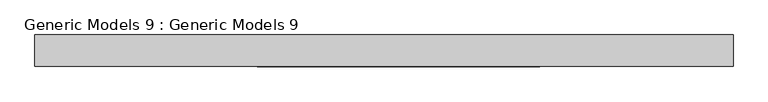
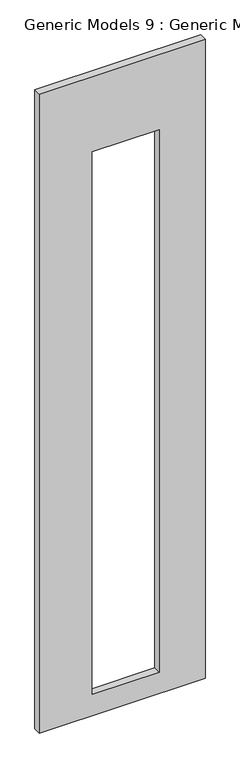
"""IFC4 building model written with IfcOpenShell, lengths in millimetres: proxy geometry, Generic Models 9 : Generic Models 9."""

from ifc_helpers import new_model, si_unit, frame, origin, place, context, project, spatial, polyline, outline, extrude, source, transform, mapped, element, save


def generic_models_9_generic_models_9_a1359b20(model_context):
    return source(origin(), model_context, "Body", "SweptSolid", [
        extrude(outline(polyline([(13668.3613642, 2250.4129028), (13668.3613642, -1141.8011568), (-152.4, -1141.8011568), (-152.4, 2250.4129028), (13668.3613642, 2250.4129028)]), holes=[polyline([(12039.6, 1310.3916602), (304.8, 1310.3916602), (304.8, -61.2083398), (12039.6, -61.2083398), (12039.6, 1310.3916602)])]), frame((0.0, -11268.8679047, 0.0), z_axis=(0.0, 1.0, 0.0), x_axis=(0.0, 0.0, 1.0)), (0.0, 0.0, 1.0), 152.4),
    ])


if __name__ == "__main__":
    model = new_model("IFC4")
    model_context = context("Model", 3, world=origin())
    ifc_project = project(units=[si_unit("LENGTHUNIT", "METRE", prefix="MILLI")], contexts=[model_context])
    site = spatial("IfcSite", under=ifc_project)
    building = spatial("IfcBuilding", under=site)
    placement = place(None, origin())
    generic_models_9_generic_models_9_shape = generic_models_9_generic_models_9_a1359b20(model_context)
    element("IfcBuildingElementProxy", 1, Name="Generic Models 9 : Generic Models 9", ObjectType="Generic Models 9 : Generic Models 9", at=placement, inside=building, context=model_context, shape_type="MappedRepresentation", body=[
        mapped(generic_models_9_generic_models_9_shape, transform((0.0, 0.0, 0.0), x_axis=(1.0, 0.0, 0.0), y_axis=(0.0, 1.0, 0.0), z_axis=(0.0, 0.0, 1.0))),
    ])
    save(model, "model.ifc")

# Revit data of these elements
# Element 1 (IfcBuildingElementProxy, "Generic Models 9 : Generic Models 9")
#   Materials on its faces: "TEAK BROWN COLOUR"
# Materials
#   "TEAK BROWN COLOUR": class "Generic", colour RGB 120 120 120, transparency 0, Cost = 0
